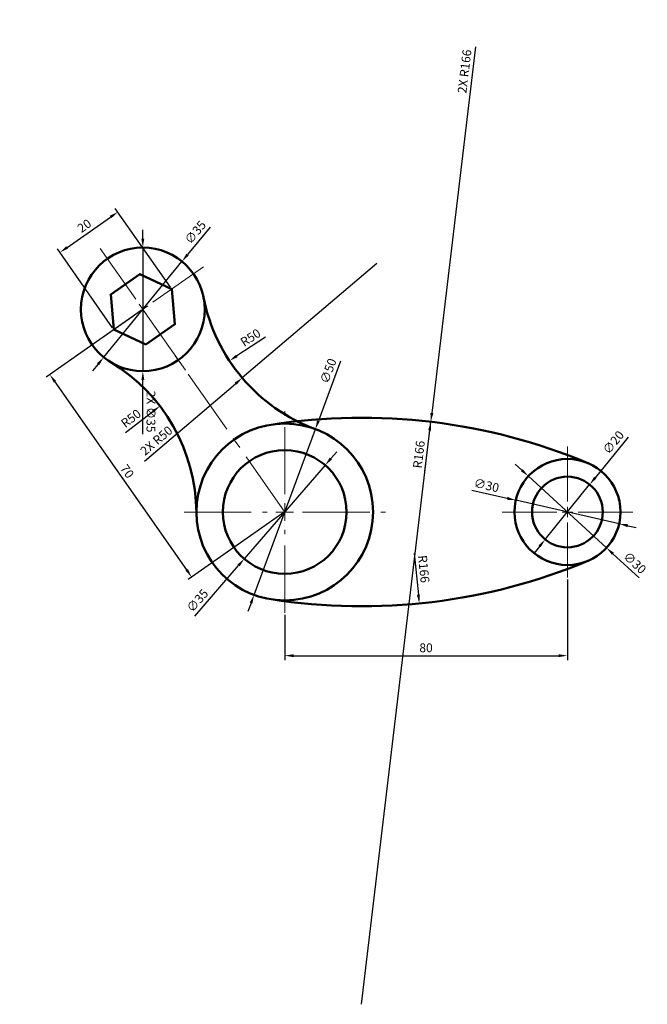
# Model space of a CAD drawing. Units: millimetres. Extents: x 9973 to 10150, y 4752 to 5030.
import ezdxf

# ---------------------------------------------------------------- set-up
doc = ezdxf.new("R2010")
doc.units = ezdxf.units.MM
doc.linetypes.add('CENTER2', pattern=[28.575, 19.05, -3.175, 3.175, -3.175])
doc.linetypes.add('HIDDENX2', pattern=[19.05, 12.7, -6.35])
doc.layers.get('Defpoints').update_dxf_attribs({"color": 3, "linetype": 'HIDDENX2'})
for name, color, linetype, lineweight in [('M-CNTR', 1, 'CENTER2', 18), ('M-DIMS', 2, 'Continuous', 25), ('M-OUTL', 7, 'Continuous', 50)]:
    doc.layers.add(name, color=color, linetype=linetype, lineweight=lineweight)
doc.styles.get("Standard").update_dxf_attribs({"font": 'arial.ttf'})
doc.dimstyles.new('ISO-25', dxfattribs={"dimtxt": 2.5, "dimasz": 2.5, "dimexe": 1.25, "dimexo": 0.625, "dimtad": 1, "dimtxsty": 'Standard', "dimcen": 2.5, "dimadec": 0, "dimazin": 0, "dimtfac": 1, "dimtmove": 0, "dimatfit": 3, "dimfxl": 1, "dimarcsym": 0})

# ---------------------------------------------------------------- blocks, each defined once
blk = doc.blocks.new('*U1')
at = {"layer": 'M-CNTR', "color": 0, "transparency": 16777216}
for p, q in [((0, 3.5), (0, 21)), ((-21, 0), (-3.5, 0)), ((3.5, 0), (21, 0)), ((0, -21), (0, -3.5))]:
    blk.add_line(p, q, dxfattribs=at)
at = {"layer": 'M-CNTR', "color": 0, "linetype": 'Continuous', "transparency": 16777216}
for p, q in [((-1.75, 0), (1.75, 0)), ((0, -1.75), (0, 1.75))]:
    blk.add_line(p, q, dxfattribs=at)
blk = doc.blocks.new('*U2')
at = {"layer": 'M-CNTR', "color": 0, "transparency": 16777216}
for p, q in [((0, 5), (0, 28.5)), ((-28.5, 0), (-5, 0)), ((5, 0), (28.5, 0)), ((0, -28.5), (0, -5))]:
    blk.add_line(p, q, dxfattribs=at)
at = {"layer": 'M-CNTR', "color": 0, "linetype": 'Continuous', "transparency": 16777216}
for p, q in [((-2.5, 0), (2.5, 0)), ((0, -2.5), (0, 2.5))]:
    blk.add_line(p, q, dxfattribs=at)
blk = doc.blocks.new('*U3')
at = {"layer": 'M-CNTR', "color": 0, "transparency": 16777216}
for p, q in [((0, 3), (0, 18.5)), ((-18.5, 0), (-3, 0)), ((3, 0), (18.5, 0)), ((0, -18.5), (0, -3))]:
    blk.add_line(p, q, dxfattribs=at)
at = {"layer": 'M-CNTR', "color": 0, "linetype": 'Continuous', "transparency": 16777216}
for p, q in [((-1.5, 0), (1.5, 0)), ((0, -1.5), (0, 1.5))]:
    blk.add_line(p, q, dxfattribs=at)
blk = doc.blocks.new('*D4')
at = {"layer": 'Defpoints', "color": 0, "transparency": 16777216}
for p in [(10127.64, 4872.52), (10047.64, 4862.52), (10127.64, 4850.36)]:
    blk.add_point(p, dxfattribs=at)
at = {"layer": 'M-DIMS', "color": 0, "lineweight": -2, "transparency": 16777216}
for p, q in [((10127.64, 4871.89), (10127.64, 4849.11)), ((10047.64, 4861.89), (10047.64, 4849.11)), ((10050.14, 4850.36), (10125.14, 4850.36))]:
    blk.add_line(p, q, dxfattribs=at)
at = {"layer": 'M-DIMS', "color": 0, "transparency": 16777216}
for points in [[(10050.14, 4850.78), (10050.14, 4849.95), (10047.64, 4850.36)], [(10125.14, 4850.78), (10125.14, 4849.95), (10127.64, 4850.36)]]:
    blk.add_solid(points, dxfattribs=at)
at = {"layer": 'M-DIMS', "color": 0, "transparency": 16777216, "insert": (10087.64, 4852.26), "char_height": 2.5, "attachment_point": 5}
blk.add_mtext('80', dxfattribs=at)
blk = doc.blocks.new('*D5')
at = {"layer": 'Defpoints', "color": 0, "transparency": 16777216}
for p in [(10000.4, 4975.92), (10015.68, 4954.09), (9999.3, 4942.62)]:
    blk.add_point(p, dxfattribs=at)
at = {"layer": 'M-DIMS', "color": 0, "lineweight": -2, "transparency": 16777216}
for p, q in [((10015.32, 4954.6), (9999.68, 4976.94)), ((9986.06, 4965.88), (9998.35, 4974.49)), ((9998.94, 4943.13), (9983.3, 4965.47))]:
    blk.add_line(p, q, dxfattribs=at)
at = {"layer": 'M-DIMS', "color": 0, "transparency": 16777216}
for points in [[(9998.11, 4974.83), (9998.59, 4974.14), (10000.4, 4975.92)], [(9985.82, 4966.22), (9986.3, 4965.54), (9984.01, 4964.45)]]:
    blk.add_solid(points, dxfattribs=at)
at = {"layer": 'M-DIMS', "color": 0, "transparency": 16777216, "insert": (9991.12, 4971.74), "char_height": 2.5, "attachment_point": 5, "rotation": 35}
blk.add_mtext('20', dxfattribs=at)
blk = doc.blocks.new('*D6')
at = {"layer": 'Defpoints', "color": 0, "transparency": 16777216}
for p in [(10007.49, 4948.36), (10047.64, 4891.02), (10021.32, 4872.59)]:
    blk.add_point(p, dxfattribs=at)
at = {"layer": 'M-DIMS', "color": 0, "lineweight": -2, "transparency": 16777216}
for p, q in [((10006.98, 4948), (9980.15, 4929.21)), ((9982.61, 4927.88), (10019.89, 4874.64)), ((10047.13, 4890.66), (10020.3, 4871.87))]:
    blk.add_line(p, q, dxfattribs=at)
at = {"layer": 'M-DIMS', "color": 0, "transparency": 16777216}
for points in [[(9982.95, 4928.12), (9982.26, 4927.64), (9981.17, 4929.93)], [(10020.23, 4874.88), (10019.55, 4874.4), (10021.32, 4872.59)]]:
    blk.add_solid(points, dxfattribs=at)
at = {"layer": 'M-DIMS', "color": 0, "transparency": 16777216, "insert": (10002.8, 4902.35), "char_height": 2.5, "attachment_point": 5, "rotation": 305}
blk.add_mtext('70', dxfattribs=at)
blk = doc.blocks.new('*D7')
at = {"layer": 'Defpoints', "color": 0, "transparency": 16777216}
for p in [(10012.31, 4920.99), (9972.64, 4890.55)]:
    blk.add_point(p, dxfattribs=at)
at = {"layer": 'M-DIMS', "color": 0, "lineweight": -2, "transparency": 16777216}
blk.add_line((10002.62, 4913.55), (10010.32, 4919.46), dxfattribs=at)
at = {"layer": 'M-DIMS', "color": 0, "transparency": 16777216}
blk.add_solid([(10010.07, 4919.8), (10010.58, 4919.13), (10012.31, 4920.99)], dxfattribs=at)
at = {"layer": 'M-DIMS', "color": 0, "transparency": 16777216, "insert": (10004.32, 4917.25), "char_height": 2.5, "attachment_point": 5, "rotation": 37.5002}
blk.add_mtext('R50', dxfattribs=at)
blk = doc.blocks.new('*D8')
at = {"layer": 'Defpoints', "color": 0, "transparency": 16777216}
for p in [(10073.73, 4961.33), (10032, 4933.79)]:
    blk.add_point(p, dxfattribs=at)
at = {"layer": 'M-DIMS', "color": 0, "lineweight": -2, "transparency": 16777216}
blk.add_line((10042.19, 4940.52), (10034.08, 4935.17), dxfattribs=at)
at = {"layer": 'M-DIMS', "color": 0, "transparency": 16777216}
blk.add_solid([(10033.85, 4935.52), (10034.31, 4934.82), (10032, 4933.79)], dxfattribs=at)
at = {"layer": 'M-DIMS', "color": 0, "transparency": 16777216, "insert": (10038.13, 4940.12), "char_height": 2.5, "attachment_point": 5, "rotation": 33.4195}
blk.add_mtext('R50', dxfattribs=at)
blk = doc.blocks.new('*D9')
at = {"layer": 'Defpoints', "color": 0, "transparency": 16777216}
for p in [(10056.31, 4914.46), (10038.97, 4867.57)]:
    blk.add_point(p, dxfattribs=at)
at = {"layer": 'M-DIMS', "color": 0, "lineweight": -2, "transparency": 16777216}
for p, q in [((10063.42, 4933.68), (10057.18, 4916.81)), ((10038.97, 4867.57), (10056.31, 4914.46)), ((10038.1, 4865.22), (10037.23, 4862.88))]:
    blk.add_line(p, q, dxfattribs=at)
at = {"layer": 'M-DIMS', "color": 0, "transparency": 16777216}
for points in [[(10056.79, 4916.95), (10057.57, 4916.66), (10056.31, 4914.46)], [(10037.71, 4865.37), (10038.49, 4865.08), (10038.97, 4867.57)]]:
    blk.add_solid(points, dxfattribs=at)
at = {"layer": 'M-DIMS', "color": 0, "transparency": 16777216, "insert": (10060.26, 4930.83), "char_height": 2.5, "attachment_point": 5, "rotation": 69.7}
blk.add_mtext('∅50', dxfattribs=at)
blk = doc.blocks.new('*D10')
at = {"layer": 'Defpoints', "color": 0, "transparency": 16777216}
for p in [(10059.08, 4904.26), (10036.2, 4877.77)]:
    blk.add_point(p, dxfattribs=at)
at = {"layer": 'M-DIMS', "color": 0, "lineweight": -2, "transparency": 16777216}
for p, q in [((10060.71, 4906.15), (10062.35, 4908.04)), ((10059.08, 4904.26), (10036.2, 4877.77)), ((10022.2, 4861.57), (10034.56, 4875.88))]:
    blk.add_line(p, q, dxfattribs=at)
at = {"layer": 'M-DIMS', "color": 0, "transparency": 16777216}
for points in [[(10060.4, 4906.42), (10061.03, 4905.88), (10059.08, 4904.26)], [(10034.25, 4876.15), (10034.88, 4875.61), (10036.2, 4877.77)]]:
    blk.add_solid(points, dxfattribs=at)
at = {"layer": 'M-DIMS', "color": 0, "transparency": 16777216, "insert": (10023.18, 4865.72), "char_height": 2.5, "attachment_point": 5, "rotation": 49.1734}
blk.add_mtext('∅35', dxfattribs=at)
blk = doc.blocks.new('*D11')
at = {"layer": 'Defpoints', "color": 0, "transparency": 16777216}
for p in [(10133.93, 4898.79), (10121.34, 4883.25)]:
    blk.add_point(p, dxfattribs=at)
at = {"layer": 'M-DIMS', "color": 0, "lineweight": -2, "transparency": 16777216}
for p, q in [((10144.8, 4912.2), (10135.51, 4900.73)), ((10121.34, 4883.25), (10133.93, 4898.79)), ((10119.77, 4881.3), (10118.2, 4879.36))]:
    blk.add_line(p, q, dxfattribs=at)
at = {"layer": 'M-DIMS', "color": 0, "transparency": 16777216}
for points in [[(10135.19, 4900.99), (10135.83, 4900.47), (10133.93, 4898.79)], [(10119.45, 4881.57), (10120.09, 4881.04), (10121.34, 4883.25)]]:
    blk.add_solid(points, dxfattribs=at)
at = {"layer": 'M-DIMS', "color": 0, "transparency": 16777216, "insert": (10140.9, 4910.51), "char_height": 2.5, "attachment_point": 5, "rotation": 50.981}
blk.add_mtext('∅20', dxfattribs=at)
blk = doc.blocks.new('*D12')
at = {"layer": 'Defpoints', "color": 0, "transparency": 16777216}
for p in [(10116.59, 4901.16), (10138.69, 4880.88)]:
    blk.add_point(p, dxfattribs=at)
at = {"layer": 'M-DIMS', "color": 0, "lineweight": -2, "transparency": 16777216}
for p, q in [((10114.74, 4902.85), (10112.9, 4904.54)), ((10116.59, 4901.16), (10138.69, 4880.88)), ((10147.94, 4872.4), (10140.54, 4879.19))]:
    blk.add_line(p, q, dxfattribs=at)
at = {"layer": 'M-DIMS', "color": 0, "transparency": 16777216}
for points in [[(10115.02, 4903.15), (10114.46, 4902.54), (10116.59, 4901.16)], [(10140.82, 4879.49), (10140.25, 4878.88), (10138.69, 4880.88)]]:
    blk.add_solid(points, dxfattribs=at)
at = {"layer": 'M-DIMS', "color": 0, "transparency": 16777216, "insert": (10146.49, 4876.4), "char_height": 2.5, "attachment_point": 5, "rotation": 317.4691}
blk.add_mtext('∅30', dxfattribs=at)
blk = doc.blocks.new('*D13')
at = {"layer": 'Defpoints', "color": 0, "transparency": 16777216}
for p in [(10018.56, 4961.91), (9996.42, 4934.8)]:
    blk.add_point(p, dxfattribs=at)
at = {"layer": 'M-DIMS', "color": 0, "lineweight": -2, "transparency": 16777216}
for p, q in [((10026.51, 4971.64), (10020.14, 4963.85)), ((9996.42, 4934.8), (10018.56, 4961.91)), ((9994.84, 4932.87), (9993.25, 4930.93))]:
    blk.add_line(p, q, dxfattribs=at)
at = {"layer": 'M-DIMS', "color": 0, "transparency": 16777216}
for points in [[(10019.82, 4964.11), (10020.46, 4963.58), (10018.56, 4961.91)], [(9994.51, 4933.13), (9995.16, 4932.6), (9996.42, 4934.8)]]:
    blk.add_solid(points, dxfattribs=at)
at = {"layer": 'M-DIMS', "color": 0, "transparency": 16777216, "insert": (10022.59, 4969.96), "char_height": 2.5, "attachment_point": 5, "rotation": 50.7547}
blk.add_mtext('∅35', dxfattribs=at)
blk = doc.blocks.new('*D14')
at = {"layer": 'Defpoints', "color": 0, "transparency": 16777216}
for p in [(10088.95, 4916.55), (10069.39, 4751.7)]:
    blk.add_point(p, dxfattribs=at)
at = {"layer": 'M-DIMS', "color": 0, "lineweight": -2, "transparency": 16777216}
blk.add_line((10087.28, 4902.48), (10088.66, 4914.06), dxfattribs=at)
at = {"layer": 'M-DIMS', "color": 0, "transparency": 16777216}
blk.add_solid([(10088.24, 4914.11), (10089.07, 4914.02), (10088.95, 4916.55)], dxfattribs=at)
at = {"layer": 'M-DIMS', "color": 0, "transparency": 16777216, "insert": (10085.93, 4907.26), "char_height": 2.5, "attachment_point": 5, "rotation": 83.2324}
blk.add_mtext('R166', dxfattribs=at)
blk = doc.blocks.new('*D15')
at = {"layer": 'Defpoints', "color": 0, "transparency": 16777216}
for p in [(10069.39, 5030.33), (10085.72, 4865.13)]:
    blk.add_point(p, dxfattribs=at)
at = {"layer": 'M-DIMS', "color": 0, "lineweight": -2, "transparency": 16777216}
blk.add_line((10084.32, 4879.23), (10085.47, 4867.62), dxfattribs=at)
at = {"layer": 'M-DIMS', "color": 0, "transparency": 16777216}
blk.add_solid([(10085.89, 4867.66), (10085.06, 4867.58), (10085.72, 4865.13)], dxfattribs=at)
at = {"layer": 'M-DIMS', "color": 0, "transparency": 16777216, "insert": (10086.67, 4874.86), "char_height": 2.5, "attachment_point": 5, "rotation": 275.6451}
blk.add_mtext('R166', dxfattribs=at)
blk = doc.blocks.new('*D16')
at = {"layer": 'Defpoints', "color": 0, "transparency": 16777216}
for p in [(10007.49, 4965.86), (10007.49, 4930.86)]:
    blk.add_point(p, dxfattribs=at)
at = {"layer": 'M-DIMS', "color": 0, "lineweight": -2, "transparency": 16777216}
for p, q in [((10007.49, 4968.36), (10007.49, 4970.86)), ((10007.49, 4965.86), (10007.49, 4930.86)), ((10007.49, 4913.01), (10007.49, 4928.36))]:
    blk.add_line(p, q, dxfattribs=at)
at = {"layer": 'M-DIMS', "color": 0, "transparency": 16777216}
for points in [[(10007.9, 4968.36), (10007.07, 4968.36), (10007.49, 4965.86)], [(10007.91, 4928.36), (10007.07, 4928.36), (10007.49, 4930.86)]]:
    blk.add_solid(points, dxfattribs=at)
at = {"layer": 'M-DIMS', "color": 0, "transparency": 16777216, "insert": (10009.46, 4919.43), "char_height": 2.5, "attachment_point": 5, "rotation": 270.0038}
blk.add_mtext('2X ∅35', dxfattribs=at)
blk = doc.blocks.new('*D17')
at = {"layer": 'Defpoints', "color": 0, "transparency": 16777216}
for p in [(10113.01, 4894.34), (10142.27, 4887.7)]:
    blk.add_point(p, dxfattribs=at)
at = {"layer": 'M-DIMS', "color": 0, "lineweight": -2, "transparency": 16777216}
for p, q in [((10100.56, 4897.17), (10110.57, 4894.89)), ((10142.27, 4887.7), (10113.01, 4894.34)), ((10144.7, 4887.14), (10147.14, 4886.59))]:
    blk.add_line(p, q, dxfattribs=at)
at = {"layer": 'M-DIMS', "color": 0, "transparency": 16777216}
for points in [[(10110.67, 4895.3), (10110.48, 4894.48), (10113.01, 4894.34)], [(10144.8, 4887.55), (10144.61, 4886.74), (10142.27, 4887.7)]]:
    blk.add_solid(points, dxfattribs=at)
at = {"layer": 'M-DIMS', "color": 0, "transparency": 16777216, "insert": (10104.67, 4898.25), "char_height": 2.5, "attachment_point": 5, "rotation": 347.2086}
blk.add_mtext('∅30', dxfattribs=at)
blk = doc.blocks.new('*D18')
at = {"layer": 'Defpoints', "color": 0, "transparency": 16777216}
for p in [(10073.73, 4961.33), (10035.63, 4928.95)]:
    blk.add_point(p, dxfattribs=at)
at = {"layer": 'M-DIMS', "color": 0, "lineweight": -2, "transparency": 16777216}
for p, q in [((10073.73, 4961.33), (10035.63, 4928.95)), ((10007.96, 4905.43), (10033.73, 4927.33))]:
    blk.add_line(p, q, dxfattribs=at)
at = {"layer": 'M-DIMS', "color": 0, "transparency": 16777216}
blk.add_solid([(10033.46, 4927.65), (10034, 4927.01), (10035.63, 4928.95)], dxfattribs=at)
at = {"layer": 'M-DIMS', "color": 0, "transparency": 16777216, "insert": (10011.54, 4910.97), "char_height": 2.5, "attachment_point": 5, "rotation": 40.3623}
blk.add_mtext('2X R50', dxfattribs=at)
blk = doc.blocks.new('*D19')
at = {"layer": 'Defpoints', "color": 0, "transparency": 16777216}
for p in [(10088.99, 4916.54), (10069.39, 4751.7)]:
    blk.add_point(p, dxfattribs=at)
at = {"layer": 'M-DIMS', "color": 0, "lineweight": -2, "transparency": 16777216}
for p, q in [((10101.6, 5022.69), (10089.28, 4919.03)), ((10069.39, 4751.7), (10088.99, 4916.54))]:
    blk.add_line(p, q, dxfattribs=at)
at = {"layer": 'M-DIMS', "color": 0, "transparency": 16777216}
blk.add_solid([(10088.87, 4919.07), (10089.69, 4918.98), (10088.99, 4916.54)], dxfattribs=at)
at = {"layer": 'M-DIMS', "color": 0, "transparency": 16777216, "insert": (10098.85, 5015.67), "char_height": 2.5, "attachment_point": 5, "rotation": 83.2205}
blk.add_mtext('2X R166', dxfattribs=at)

msp = doc.modelspace()

# ---------------------------------------------------------------- linework, layer by layer
at = {"layer": 'M-CNTR'}
msp.add_line((10047.639, 4891.016), (10007.489, 4948.357), dxfattribs=at)
at = {"layer": 'M-OUTL'}
msp.add_lwpolyline([(10008.36, 4938.395), (10016.552, 4944.131), (10015.68, 4954.093), (10006.617, 4958.319), (9998.426, 4952.583), (9999.297, 4942.621)], close=True, dxfattribs=at)
for centre, radius in [((10007.489, 4948.357), 17.5), ((10047.639, 4891.016), 25), ((10047.639, 4891.016), 17.5), ((10127.639, 4891.016), 15), ((10127.639, 4891.016), 10)]:
    msp.add_circle(centre, radius, dxfattribs=at)
for centre, radius, start, end in [((10073.73, 4961.332), 50, 191.08235, 249.64238), ((9972.641, 4890.548), 50, 0.35762, 58.91765), ((10069.389, 4751.704), 166, 67.30897, 98.87361), ((10069.389, 5030.329), 166, 261.12639, 292.69103)]:
    msp.add_arc(centre, radius, start, end, dxfattribs=at)

# ---------------------------------------------------------------- block references
at = {"layer": 'M-CNTR', "rotation": 304.9999999999995}
msp.add_blockref('*U1', (10007.489, 4948.357), dxfattribs=at)
at = {"layer": 'M-CNTR'}
for name, p in [('*U2', (10047.639, 4891.016)), ('*U3', (10127.639, 4891.016))]:
    msp.add_blockref(name, p, dxfattribs=at)

# ---------------------------------------------------------------- dimensions: what is measured, and where the dimension line sits
at = {"layer": 'M-DIMS'}
for center, mpoint, picture, middle in [((10069.389, 5030.329), (10085.718, 4865.134), '*D15', (10084.775, 4874.67)), ((10073.73, 4961.332), (10031.997, 4933.794), '*D8', (10039.181, 4938.534)), ((9972.641, 4890.548), (10012.308, 4920.986), '*D7', (10005.479, 4915.746)), ((10069.389, 4751.704), (10088.951, 4916.547), '*D14', (10087.822, 4907.032))]:
    dim = msp.add_radius_dim(center=center, mpoint=mpoint, dimstyle='ISO-25', override={"dimclrd": 0, "dimclre": 0, "dimclrt": 0}, dxfattribs=at)
    dim.commit()
    dim.dimension.update_dxf_attribs({"geometry": picture, "text_midpoint": middle, "dimtype": 164})
for center, mpoint, picture, middle in [((10069.389, 4751.704), (10088.985, 4916.543), '*D19', (10100.743, 5015.447)), ((10073.73, 4961.332), (10035.632, 4928.951), '*D18', (10012.773, 4909.522))]:
    dim = msp.add_radius_dim(center=center, mpoint=mpoint, text='2X <>', dimstyle='ISO-25', override={"dimdec": 0, "dimlfac": 1, "dimrnd": 0, "dimzin": 0, "dimdsep": 46, "dimlunit": 2}, dxfattribs=at)
    dim.commit()
    dim.dimension.update_dxf_attribs({"geometry": picture, "text_midpoint": middle, "dimtype": 164})
dim = msp.add_aligned_dim(p1=(9999.297, 4942.621), p2=(10015.68, 4954.093), distance=26.645, dimstyle='ISO-25', override={"dimclrd": 0, "dimclre": 0, "dimclrt": 0}, dxfattribs=at)
dim.commit()
dim.dimension.update_dxf_attribs({"geometry": '*D5', "text_midpoint": (9991.115, 4971.741)})
for p1, p2, picture, middle in [((9996.418, 4934.804), (10018.56, 4961.91), '*D13', (10022.591, 4969.96)), ((10116.586, 4901.156), (10138.693, 4880.877), '*D12', (10146.489, 4876.4))]:
    dim = msp.add_diameter_dim_2p(p1=p1, p2=p2, dimstyle='ISO-25', override={"dimclrd": 0, "dimclre": 0, "dimclrt": 0}, dxfattribs=at)
    dim.commit()
    dim.dimension.update_dxf_attribs({"geometry": picture, "text_midpoint": middle})
dim = msp.add_diameter_dim_2p(p1=(10007.488, 4965.857), p2=(10007.49, 4930.857), text='2X <>', dimstyle='ISO-25', override={"dimdec": 0, "dimlfac": 1, "dimrnd": 0, "dimzin": 0, "dimdsep": 46, "dimlunit": 2}, dxfattribs=at)
dim.commit()
dim.dimension.update_dxf_attribs({"geometry": '*D16', "text_midpoint": (10007.491, 4919.431), "dimtype": 163})
dim = msp.add_linear_dim(base=(10021.322, 4872.589), p1=(10007.489, 4948.357), p2=(10047.639, 4891.016), angle=305, dimstyle='ISO-25', override={"dimclrd": 0, "dimclre": 0, "dimclrt": 0}, dxfattribs=at)
dim.commit()
dim.dimension.update_dxf_attribs({"geometry": '*D6', "text_midpoint": (10001.247, 4901.259), "dimtype": 161})
for p1, p2, override, picture, middle in [((10038.966, 4867.569), (10056.313, 4914.464), {"dimclrd": 0, "dimclre": 0, "dimclrt": 0}, '*D9', (10062.112, 4930.141)), ((10121.343, 4883.247), (10133.935, 4898.786), {"dimclrd": 0, "dimclre": 0, "dimclrt": 0}, '*D11', (10142.428, 4909.266)), ((10059.08, 4904.258), (10036.198, 4877.774), {"dimclrd": 0, "dimclre": 0, "dimclrt": 0}, '*D10', (10024.672, 4864.433)), ((10142.267, 4887.695), (10113.011, 4894.337), {"dimdec": 0, "dimlfac": 1, "dimrnd": 0, "dimzin": 0, "dimdsep": 46, "dimlunit": 2}, '*D17', (10104.235, 4896.33))]:
    dim = msp.add_diameter_dim_2p(p1=p1, p2=p2, dimstyle='ISO-25', override=override, dxfattribs=at)
    dim.commit()
    dim.dimension.update_dxf_attribs({"geometry": picture, "text_midpoint": middle, "dimtype": 163})
dim = msp.add_linear_dim(base=(10127.639, 4850.362), p1=(10047.639, 4862.516), p2=(10127.639, 4872.516), dimstyle='ISO-25', override={"dimclrd": 0, "dimclre": 0, "dimclrt": 0}, dxfattribs=at)
dim.commit()
dim.dimension.update_dxf_attribs({"geometry": '*D4', "text_midpoint": (10087.639, 4852.263)})

doc.saveas('drawing.dxf')
